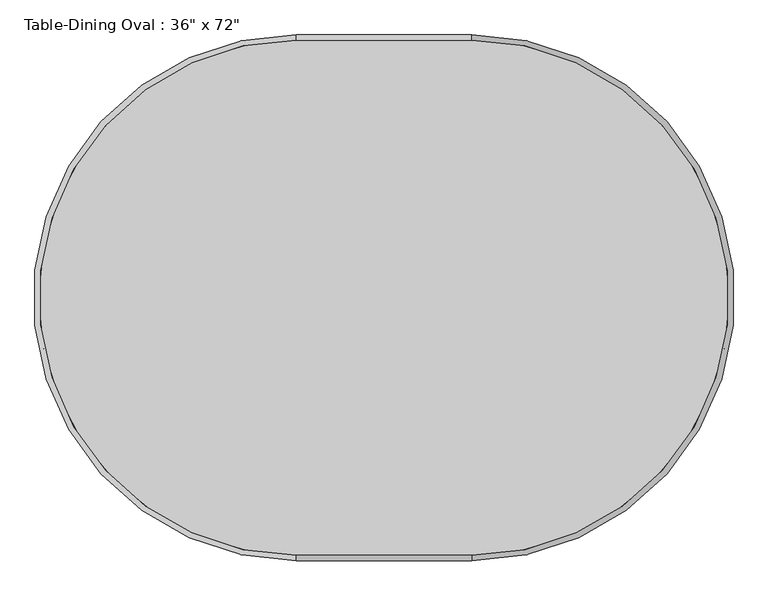
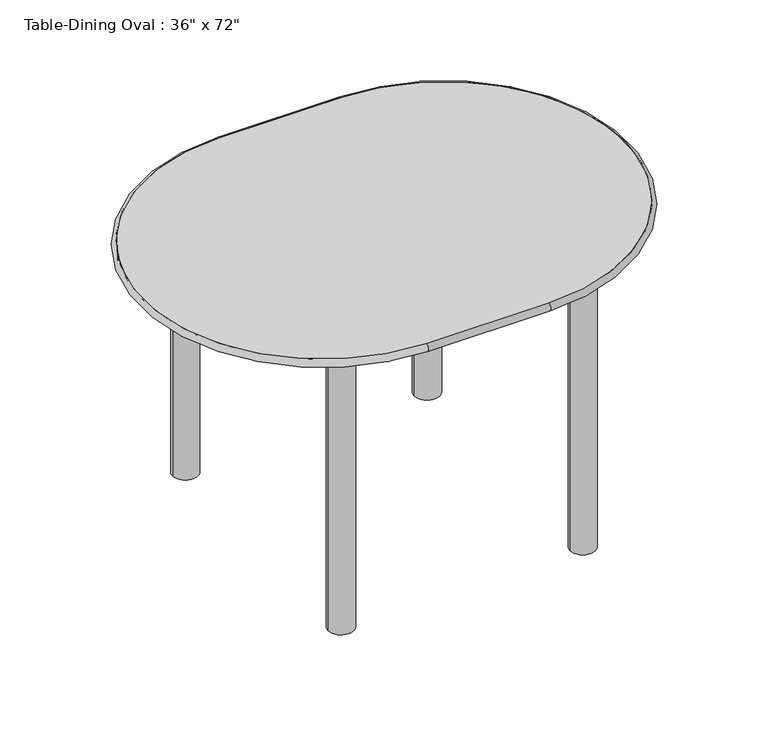
"""IFC4 building model written with IfcOpenShell, lengths in millimetres: furniture geometry."""

from ifc_helpers import new_model, si_unit, point, frame, frame_2d, origin, origin_with_axes, place, context, project, spatial, polyline, circle_curve, ellipse_curve, trimmed, segment, composite_curve, outline, extrude, source, transform, mapped, element, save
from ifc_brep_helpers import plane_surface, cylinder_surface, revolved_surface, advanced_brep


def furniture_be1c6672(model_context):
    return source(origin(), model_context, "Body", "SolidModel", [
        advanced_brep(
        [(-554.2196721, -805.7733607, 762.0), (-554.2196721, -805.7733607, 742.95), (-249.4196721, -805.7733607, 742.95), (-249.4196721, -805.7733607, 762.0), (-249.4196721, 89.5766393, 762.0), (-249.4196721, 89.5766393, 742.95), (-554.2196721, 89.5766393, 742.95), (-554.2196721, 89.5766393, 762.0)],
        [
            (0, 1, circle_curve(frame((-554.2196721, -805.7733607, 752.475), z_axis=(1.0, 0.0, 0.0), x_axis=(0.0, 1.0, 0.0)), 9.525)),
            (1, 2),
            (2, 3, circle_curve(frame((-249.4196721, -805.7733607, 752.475), z_axis=(-1.0, 0.0, 0.0), x_axis=(0.0, 1.0, 0.0)), 9.525)),
            (3, 0),
            (1, 0),
            (3, 2),
            (4, 3, circle_curve(frame((-249.4196721, -358.0983607, 762.0), z_axis=(0.0, 0.0, -1.0), x_axis=(0.0, -1.0, 0.0)), 447.675)),
            (2, 5, circle_curve(frame((-249.4196721, -358.0983607, 742.95), z_axis=(0.0, 0.0, 1.0), x_axis=(0.0, -1.0, 0.0)), 447.675)),
            (5, 4, circle_curve(frame((-249.4196721, 89.5766393, 752.475), z_axis=(1.0, 0.0, 0.0), x_axis=(0.0, -1.0, 0.0)), 9.525)),
            (4, 5),
            (5, 6),
            (6, 7, circle_curve(frame((-554.2196721, 89.5766393, 752.475), z_axis=(1.0, 0.0, 0.0), x_axis=(0.0, -1.0, 0.0)), 9.525)),
            (7, 4),
            (7, 6),
            (0, 7, circle_curve(frame((-554.2196721, -358.0983607, 762.0), z_axis=(0.0, 0.0, -1.0), x_axis=(0.0, 1.0, 0.0)), 447.675)),
            (6, 1, circle_curve(frame((-554.2196721, -358.0983607, 742.95), z_axis=(0.0, 0.0, 1.0), x_axis=(0.0, 1.0, 0.0)), 447.675)),
        ],
        [
            cylinder_surface(frame((-554.2196721, -805.7733607, 752.475), z_axis=(-1.0, 0.0, 0.0), x_axis=(0.0, 1.0, 0.0)), 9.525),
            plane_surface(frame((-554.2196721, -805.7733607, 762.0), z_axis=(0.0, 1.0, 0.0), x_axis=(1.0, 0.0, 0.0))),
            revolved_surface(trimmed(ellipse_curve(frame((-249.4196721, -805.7733607, 752.475), z_axis=(-1.0, 0.0, 0.0), x_axis=(0.0, 1.0, 0.0)), 9.525, 9.525), [point((-249.4196721, -805.7733607, 742.95))], [point((-249.4196721, -805.7733607, 762.0))], True, "CARTESIAN"), (-249.4196721, -358.0983607, 0.0), (0.0, 0.0, 1.0)),
            revolved_surface(polyline([(-249.4196721, -805.7733607, 762.0), (-249.4196721, -805.7733607, 742.95)]), (-249.4196721, -358.0983607, 0.0), (0.0, 0.0, 1.0)),
            cylinder_surface(frame((-249.4196721, 89.5766393, 752.475), z_axis=(1.0, 0.0, 0.0), x_axis=(0.0, -1.0, 0.0)), 9.525),
            plane_surface(frame((-249.4196721, 89.5766393, 762.0), z_axis=(0.0, -1.0, 0.0), x_axis=(-1.0, 0.0, 0.0))),
            revolved_surface(trimmed(ellipse_curve(frame((-554.2196721, 89.5766393, 752.475), z_axis=(1.0, 0.0, 0.0), x_axis=(0.0, -1.0, 0.0)), 9.525, 9.525), [point((-554.2196721, 89.5766393, 742.95))], [point((-554.2196721, 89.5766393, 762.0))], True, "CARTESIAN"), (-554.2196721, -358.0983607, 0.0), (0.0, 0.0, 1.0)),
            revolved_surface(polyline([(-554.2196721, 89.57663930000001, 762.0), (-554.2196721, 89.57663930000001, 742.95)]), (-554.2196721, -358.0983607, 0.0), (0.0, 0.0, 1.0)),
        ],
        [
            (0, [[1, 2, 3, 4]]),
            (1, [[5, -4, 6, -2]]),
            (2, [[7, -3, 8, 9]]),
            (3, [[-8, -6, -7, 10]]),
            (4, [[-9, 11, 12, 13]]),
            (5, [[-10, -13, 14, -11]]),
            (6, [[15, -12, 16, -1]]),
            (7, [[-16, -14, -15, -5]]),
        ],
    ),
        extrude(outline(composite_curve([segment(trimmed(circle_curve(frame_2d((-703.4446721, -21.5483607)), 31.75), [point((-735.1946721, -21.5483607))], [point((-671.6946721, -21.5483607))], False, "CARTESIAN"), True, "CONTINUOUS"), segment(trimmed(circle_curve(frame_2d((-703.4446721, -21.5483607)), 31.75), [point((-671.6946721, -21.5483607))], [point((-735.1946721, -21.5483607))], False, "CARTESIAN"), True, "CONTINUOUS")], self_intersect=False)), origin_with_axes(), (0.0, 0.0, 1.0), 742.95),
        extrude(outline(composite_curve([segment(trimmed(circle_curve(frame_2d((-703.4446721, -694.6483607)), 31.75), [point((-735.1946721, -694.6483607))], [point((-671.6946721, -694.6483607))], False, "CARTESIAN"), True, "CONTINUOUS"), segment(trimmed(circle_curve(frame_2d((-703.4446721, -694.6483607)), 31.75), [point((-671.6946721, -694.6483607))], [point((-735.1946721, -694.6483607))], False, "CARTESIAN"), True, "CONTINUOUS")], self_intersect=False)), origin_with_axes(), (0.0, 0.0, 1.0), 742.95),
        extrude(outline(composite_curve([segment(trimmed(circle_curve(frame_2d((-100.1946721, -21.5483607)), 31.75), [point((-131.9446721, -21.5483607))], [point((-68.4446721, -21.5483607))], False, "CARTESIAN"), True, "CONTINUOUS"), segment(trimmed(circle_curve(frame_2d((-100.1946721, -21.5483607)), 31.75), [point((-68.4446721, -21.5483607))], [point((-131.9446721, -21.5483607))], False, "CARTESIAN"), True, "CONTINUOUS")], self_intersect=False)), origin_with_axes(), (0.0, 0.0, 1.0), 742.95),
        extrude(outline(composite_curve([segment(trimmed(circle_curve(frame_2d((-100.1946721, -694.6483607)), 31.75), [point((-131.9446721, -694.6483607))], [point((-68.4446721, -694.6483607))], False, "CARTESIAN"), True, "CONTINUOUS"), segment(trimmed(circle_curve(frame_2d((-100.1946721, -694.6483607)), 31.75), [point((-68.4446721, -694.6483607))], [point((-131.9446721, -694.6483607))], False, "CARTESIAN"), True, "CONTINUOUS")], self_intersect=False)), origin_with_axes(), (0.0, 0.0, 1.0), 742.95),
        extrude(outline(polyline([(-81.1446721, -2.4983607), (-81.1446721, -713.6983607), (-722.4946721, -713.6983607), (-722.4946721, -2.4983607), (-81.1446721, -2.4983607)]), holes=[polyline([(-100.1946721, -21.5483607), (-703.4446721, -21.5483607), (-703.4446721, -694.6483607), (-100.1946721, -694.6483607), (-100.1946721, -21.5483607)])]), frame((0.0, 0.0, 692.15), z_axis=(0.0, 0.0, 1.0), x_axis=(1.0, 0.0, 0.0)), (0.0, 0.0, 1.0), 50.8),
        extrude(outline(composite_curve([segment(polyline([(-554.2196721, 89.5766393), (-249.4196721, 89.5766393)]), True, "CONTINUOUS"), segment(trimmed(circle_curve(frame_2d((-249.4196721, -358.0983607)), 447.675), [point((-249.4196721, 89.5766393))], [point((198.2553279, -358.0983607))], False, "CARTESIAN"), True, "CONTINUOUS"), segment(trimmed(circle_curve(frame_2d((-249.4196721, -358.0983607)), 447.675), [point((198.2553279, -358.0983607))], [point((-249.4196721, -805.7733607))], False, "CARTESIAN"), True, "CONTINUOUS"), segment(polyline([(-249.4196721, -805.7733607), (-554.2196721, -805.7733607)]), True, "CONTINUOUS"), segment(trimmed(circle_curve(frame_2d((-554.2196721, -358.0983607)), 447.675), [point((-554.2196721, -805.7733607))], [point((-1001.8946721, -358.0983607))], False, "CARTESIAN"), True, "CONTINUOUS"), segment(trimmed(circle_curve(frame_2d((-554.2196721, -358.0983607)), 447.675), [point((-1001.8946721, -358.0983607))], [point((-554.2196721, 89.5766393))], False, "CARTESIAN"), True, "CONTINUOUS")], self_intersect=False)), frame((0.0, 0.0, 742.95), z_axis=(0.0, 0.0, 1.0), x_axis=(1.0, 0.0, 0.0)), (0.0, 0.0, 1.0), 19.05),
    ])


if __name__ == "__main__":
    model = new_model("IFC4")
    model_context = context("Model", 3, world=origin())
    ifc_project = project(units=[si_unit("LENGTHUNIT", "METRE", prefix="MILLI")], contexts=[model_context])
    site = spatial("IfcSite", under=ifc_project)
    building = spatial("IfcBuilding", under=site)
    placement = place(None, origin())
    furniture_shape = furniture_be1c6672(model_context)
    element("IfcFurniture", 1, ObjectType="Table-Dining Oval : 36\" x 72\"", at=placement, inside=building, context=model_context, shape_type="MappedRepresentation", body=[
        mapped(furniture_shape, transform((0.0, 0.0, 0.0), x_axis=(1.0, 0.0, 0.0), y_axis=(0.0, 1.0, 0.0), z_axis=(0.0, 0.0, 1.0))),
    ])
    save(model, "model.ifc")

# Revit data of these elements
# Type "Table-Dining Oval : 36\" x 72\""
#   Assembly Code = "E2020200"
#   Length = 4' - 0"
#   Width = 3' - 0"
#   Base Material = Steel, Chrome Plated
#   Top Material = Glass - Clear, Grey
#   Default Elevation = 0
#   Description = (empty or 0)
# Element 1 (IfcFurniture, "Table-Dining Oval : 36\" x 72\"")
#   Materials on its faces: "Steel, Chrome Plated", "Glass - Clear, Grey"
# Materials
#   "Steel, Chrome Plated": class "Metal", colour RGB 17 17 17, transparency 0, Description = "Chromiuim plated steel", Cost = 0
#   "Glass - Clear, Grey": class "Glass", colour RGB 252 255 255, transparency 0.64
